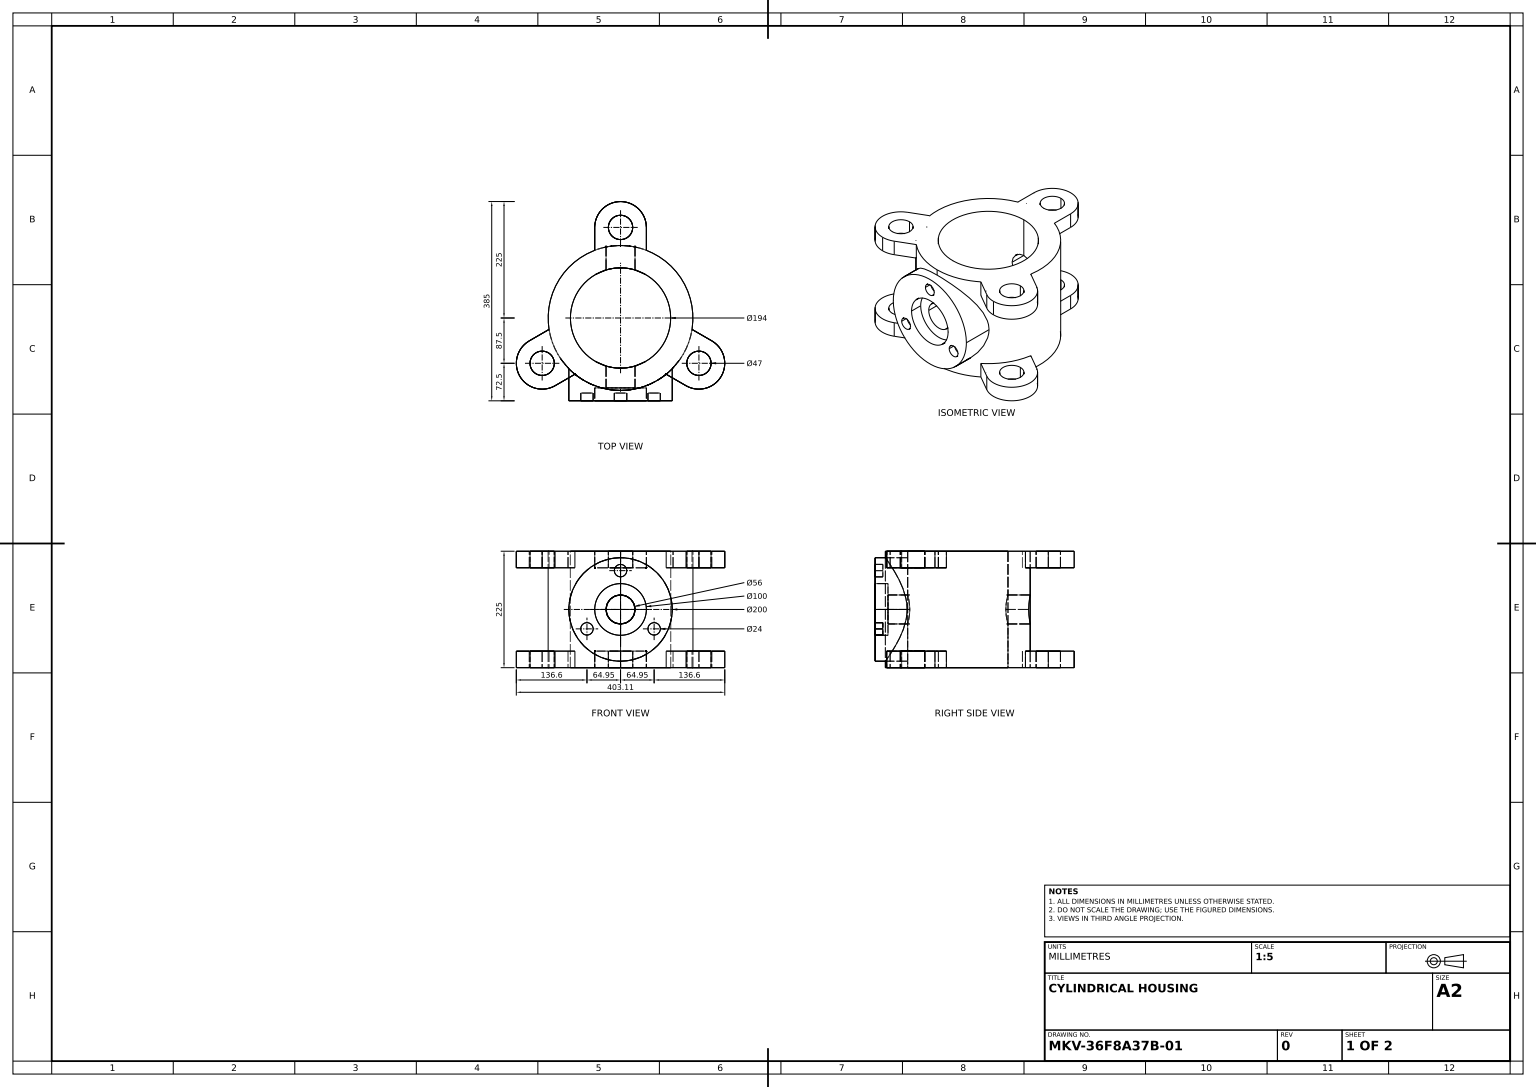
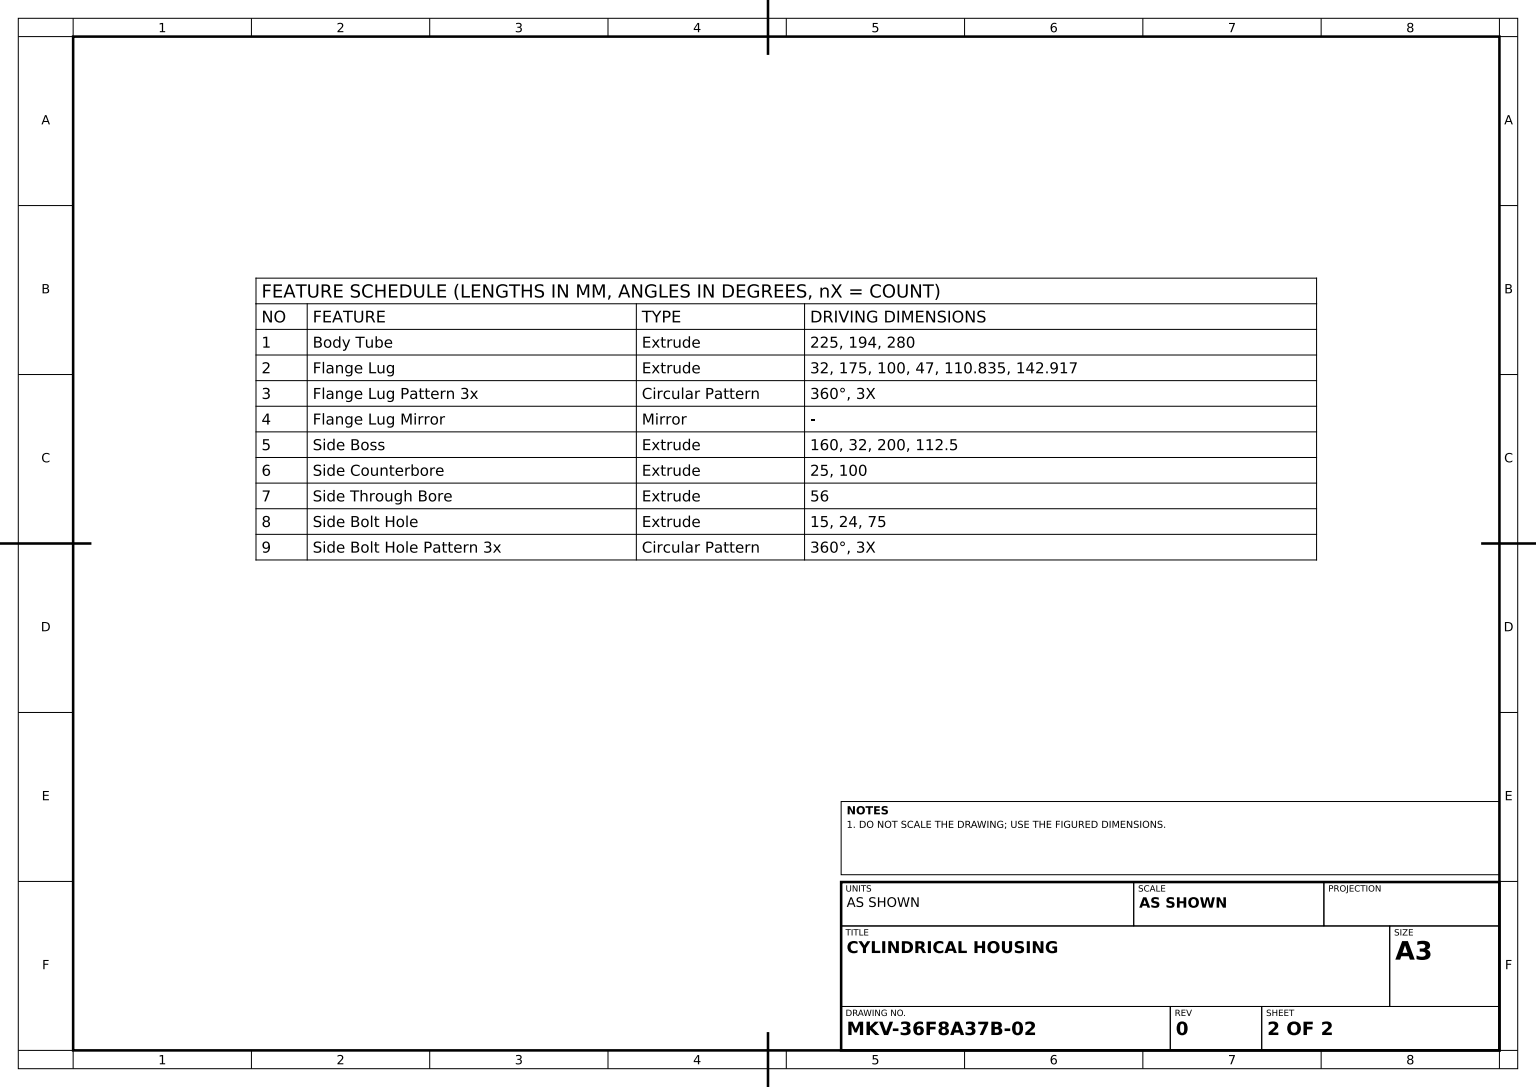
from build123d import *

# Parameters (mm, degrees)
BODY_TUBE_SKETCH_R                = 140
BODY_TUBE_SKETCH_R_2              = 97
BODY_TUBE_DEPTH                   = 225
FLANGE_LUG_SKETCH_R               = 23.5
FLANGE_LUG_DEPTH                  = 32
FLANGE_LUG_PATTERN_3X_COUNT       = 3
FLANGE_LUG_MIRROR_COPY_1_SKETCH_R = 23.5
FLANGE_LUG_MIRROR_COPY_1_DEPTH    = 32
FLANGE_LUG_MIRROR_COPY_2_SKETCH_R = 23.5
FLANGE_LUG_MIRROR_COPY_2_DEPTH    = 32
FLANGE_LUG_MIRROR_COPY_3_SKETCH_R = 23.5
FLANGE_LUG_MIRROR_COPY_3_DEPTH    = 32
SIDE_BOSS_REACH                   = 491.361
SIDE_BOSS_END_RADIUS              = 140
SIDE_BOSS_SKETCH_R                = 100
SIDE_COUNTERBORE_SKETCH_R         = 50
SIDE_COUNTERBORE_DEPTH            = 25
SIDE_BORE_SKETCH_R                = 28
SIDE_THROUGH_BORE_DEPTH           = 470.945948606
SIDE_BOLT_HOLE_SKETCH_R           = 12
SIDE_BOLT_HOLE_DEPTH              = 15
SIDE_BOLT_HOLE_PATTERN_3X_COUNT   = 3


with BuildPart() as part:
    # Body Tube Sketch → Body Tube (new body)
    with BuildSketch(Plane(origin=(0, 0, 0), x_dir=(1, 0, 0), z_dir=(0, 1, 0))):
        with Locations(Location((0, 0, 0), (0, 0, 270))):
            Circle(BODY_TUBE_SKETCH_R)
        with Locations(Location((0, 0, 0), (0, 0, 270))):
            Circle(BODY_TUBE_SKETCH_R_2, mode=Mode.SUBTRACT)
    body_tube = extrude(amount=BODY_TUBE_DEPTH)

    # Flange Lug Sketch → Flange Lug (add)
    with BuildSketch(Plane(origin=(0, 225, 0), x_dir=(1, 0, 0), z_dir=(0, 1, 0))):
        with BuildLine():
            Line((-50, 175), (-50, 110.834659577))
            Line((-50, 110.834659577), (50, 110.834659577))
            Line((50, 110.834659577), (50, 175))
            ThreePointArc((50, 175), (0, 225), (-50, 175))
        make_face()
        with Locations(Location((0, 175, 0), (0, 0, 270))):
            Circle(FLANGE_LUG_SKETCH_R, mode=Mode.SUBTRACT)
    flange_lug = extrude(amount=-FLANGE_LUG_DEPTH)

    # Flange Lug Pattern 3x: Flange Lug ×3 about axis
    flange_lug_pattern_3x_axis = Axis((0, 0, 0), (0, 1, 0))
    for i in range(1, FLANGE_LUG_PATTERN_3X_COUNT):
        add(flange_lug.rotate(flange_lug_pattern_3x_axis, i * 360 / FLANGE_LUG_PATTERN_3X_COUNT))

    # Flange Lug Mirror: Body Tube across plane
    add(body_tube.mirror(Plane.ZX.offset(112.5)))

    # Flange Lug Mirror copy 1 sketch → Flange Lug Mirror copy 1 (add)
    with BuildSketch(Plane(origin=(0, 0, 0), x_dir=(-0.4999999999999998, 0, -0.8660254037844387), z_dir=(0, -1, 0))):
        with BuildLine():
            Line((-50, -175), (-50, -110.834659577))
            Line((-50, -110.834659577), (50, -110.834659577))
            Line((50, -110.834659577), (50, -175))
            ThreePointArc((50, -175), (0, -225), (-50, -175))
        make_face()
        with Locations((0, -175)):
            Circle(FLANGE_LUG_MIRROR_COPY_1_SKETCH_R, mode=Mode.SUBTRACT)
    extrude(amount=-FLANGE_LUG_MIRROR_COPY_1_DEPTH)

    # Flange Lug Mirror copy 2 sketch → Flange Lug Mirror copy 2 (add)
    with BuildSketch(Plane(origin=(0, 0, 0), x_dir=(-0.5000000000000004, 0, 0.8660254037844384), z_dir=(0, -1, 0))):
        with BuildLine():
            Line((-50, -175), (-50, -110.834659577))
            Line((-50, -110.834659577), (50, -110.834659577))
            Line((50, -110.834659577), (50, -175))
            ThreePointArc((50, -175), (0, -225), (-50, -175))
        make_face()
        with Locations((0, -175)):
            Circle(FLANGE_LUG_MIRROR_COPY_2_SKETCH_R, mode=Mode.SUBTRACT)
    extrude(amount=-FLANGE_LUG_MIRROR_COPY_2_DEPTH)

    # Flange Lug Mirror copy 3 sketch → Flange Lug Mirror copy 3 (add)
    with BuildSketch(Plane.XZ):
        with BuildLine():
            Line((-50, -175), (-50, -110.834659577))
            Line((-50, -110.834659577), (50, -110.834659577))
            Line((50, -110.834659577), (50, -175))
            ThreePointArc((50, -175), (0, -225), (-50, -175))
        make_face()
        with Locations((0, -175)):
            Circle(FLANGE_LUG_MIRROR_COPY_3_SKETCH_R, mode=Mode.SUBTRACT)
    extrude(amount=-FLANGE_LUG_MIRROR_COPY_3_DEPTH)

    # Side Boss: up to this cylinder (the profile starts outside it)
    side_boss_end = Plane(origin=(0, 112.5, 0), z_dir=(0, -1, 0)) * Cylinder(SIDE_BOSS_END_RADIUS, 1263.722, mode=Mode.PRIVATE)
    # Side Boss Sketch → Side Boss (add, up to the surface)
    with BuildSketch(Plane.XY.offset(160), mode=Mode.PRIVATE) as side_boss_sk1:
        with Locations((0, 112.5)):
            Circle(SIDE_BOSS_SKETCH_R)
    side_boss_tool1 = extrude(side_boss_sk1.sketch, amount=-SIDE_BOSS_REACH, mode=Mode.PRIVATE) - side_boss_end
    add(side_boss_tool1.solids().sort_by_distance((0, 112.5, 160))[0])

    # Side Counterbore Sketch → Side Counterbore (cut)
    with BuildSketch(Plane.XY.offset(160)):
        with Locations((0, 112.5)):
            Circle(SIDE_COUNTERBORE_SKETCH_R)
    extrude(amount=-SIDE_COUNTERBORE_DEPTH, mode=Mode.SUBTRACT)

    # Side Bore Sketch → Side Through Bore (cut, through all)
    with BuildSketch(Plane.XY.offset(135)):
        with Locations((0, 112.5)):
            Circle(SIDE_BORE_SKETCH_R)
    extrude(amount=-SIDE_THROUGH_BORE_DEPTH, mode=Mode.SUBTRACT)

    # Side Bolt Hole Sketch → Side Bolt Hole (cut)
    with BuildSketch(Plane.XY.offset(160)):
        with Locations((0, 187.5)):
            Circle(SIDE_BOLT_HOLE_SKETCH_R)
    side_bolt_hole = extrude(amount=-SIDE_BOLT_HOLE_DEPTH, mode=Mode.SUBTRACT)

    # Side Bolt Hole Pattern 3x: Side Bolt Hole ×3 about axis
    side_bolt_hole_pattern_3x_axis = Axis((0, 112.5, 0), (0, 0, 1))
    for i in range(1, SIDE_BOLT_HOLE_PATTERN_3X_COUNT):
        add(side_bolt_hole.rotate(side_bolt_hole_pattern_3x_axis, i * 360 / SIDE_BOLT_HOLE_PATTERN_3X_COUNT), mode=Mode.SUBTRACT)


solid = part.part
